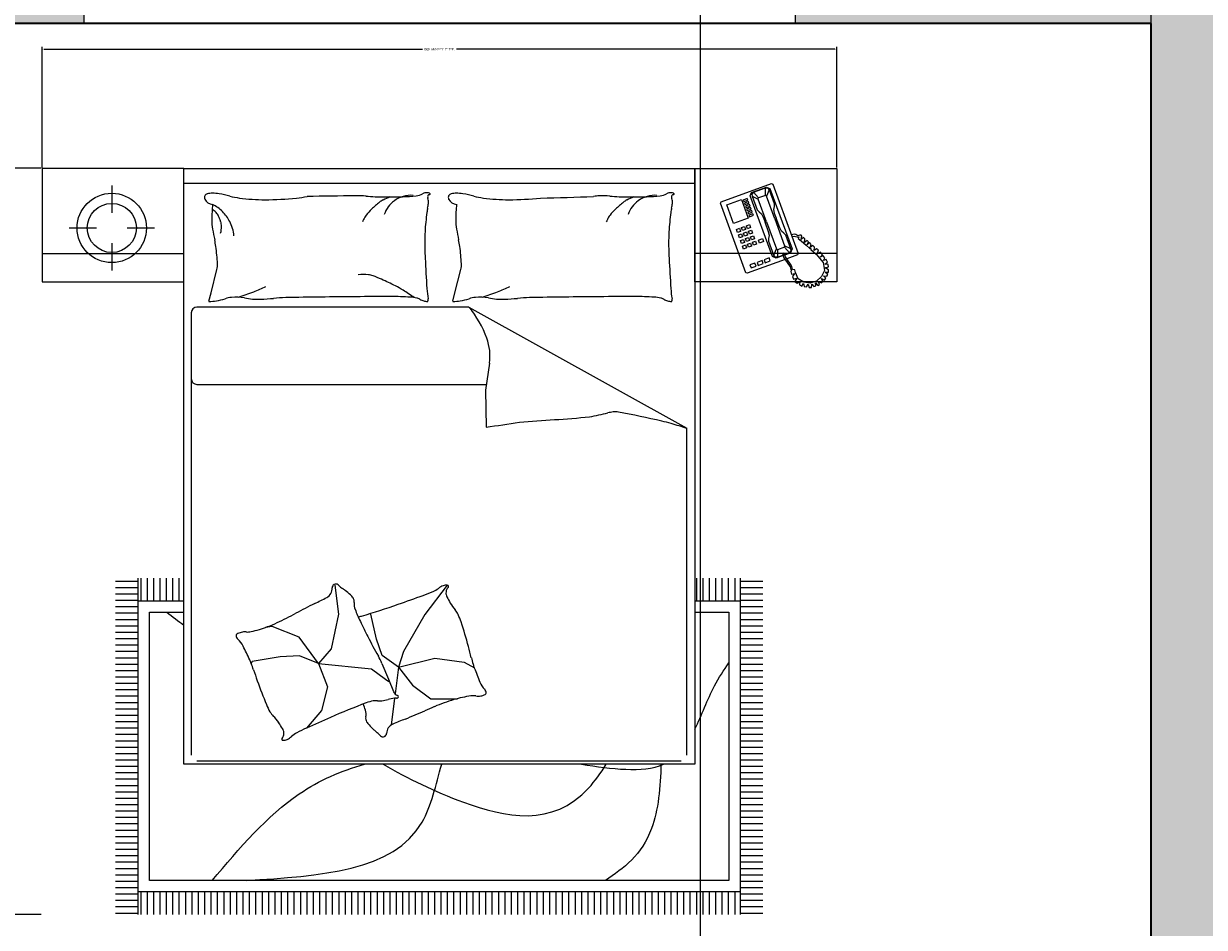
# Model space of a CAD drawing. Units: inches. Extents: x 311 to 815, y -527 to 136.
# Tile 19 of 21: x 444 to 544, y -63 to 13. Entities that reach past the tile are written whole.
import ezdxf

# ---------------------------------------------------------------- set-up
doc = ezdxf.new("R2010")
doc.units = ezdxf.units.IN
doc.header["$MEASUREMENT"] = 0
for name, color, linetype, lineweight in [('A-ANNO-DIMS', 1, 'Continuous', 18), ('A-WALL-PATT', 242, 'Continuous', 13), ('wall', 1, 'Continuous', 35), ('win', 5, 'Continuous', 18)]:
    doc.layers.add(name, color=color, linetype=linetype, lineweight=lineweight)
doc.layers.add('furniture', color=50, linetype='Continuous', lineweight=13, transparency=0.8)
doc.styles.add('DIM_FONT', font='SIMPLEX.shx', dxfattribs={"width": 0.8})
doc.styles.get("Standard").update_dxf_attribs({"font": 'arial.ttf'})
doc.dimstyles.get("Standard").update_dxf_attribs({"dimtxt": 0.18, "dimasz": 0.18, "dimexe": 0.18, "dimexo": 0.0625, "dimgap": 0.09, "dimtad": 0, "dimtih": 1, "dimtoh": 1, "dimdec": 1, "dimzin": 0, "dimdsep": 46, "dimlunit": 4, "dimtxsty": 'Standard', "dimcen": 0.09, "dimadec": 0, "dimazin": 0, "dimtfac": 1, "dimtdec": 1, "dimtofl": 0, "dimtmove": 0, "dimatfit": 3, "dimfxl": 1, "dimtolj": 1, "dimtzin": 0, "dimarcsym": 0})

# ---------------------------------------------------------------- blocks, each defined once
blk = doc.blocks.new('A$C4F634EDD')
for p, q in [((0, 2.6295), (0, 2.2295)), ((0.5, 2.6295), (0, 2.6295)), ((0.5, 2.6295), (2.3, 2.6295)), ((0.5, 0.5295), (0.5, 2.6295)), ((0.5, 2.2295), (0.5, 2.6295)), ((2.3, 2.6295), (2.3, 0.5295)), ((2.3, 2.6295), (2.8, 2.6295)), ((2.3, 2.2295), (2.3, 2.6295)), ((2.8, 2.6295), (2.8, 2.2295)), ((0.2457, 2.5697), (0.2457, 2.4733)), ((0.5, 2.5771), (2.3, 2.5771)), ((2.392, 2.5115), (2.5692, 2.5765)), ((2.4946, 2.5331), (2.4985, 2.5445)), ((2.4985, 2.5445), (2.5516, 2.564)), ((2.5062, 2.5454), (2.5004, 2.5392)), ((2.5004, 2.5392), (2.5013, 2.5315)), ((2.5062, 2.5454), (2.5487, 2.561)), ((2.5235, 2.5256), (2.5062, 2.5454)), ((2.5483, 2.5347), (2.5487, 2.561)), ((2.5487, 2.561), (2.5571, 2.56)), ((2.5615, 2.5536), (2.5514, 2.5318)), ((2.5516, 2.564), (2.5637, 2.5584)), ((2.5571, 2.56), (2.5615, 2.5536)), ((2.5615, 2.5536), (2.5791, 2.5058)), ((2.5637, 2.5584), (2.6418, 2.3458)), ((2.5692, 2.5765), (2.574, 2.5743)), ((2.574, 2.5743), (2.6638, 2.3298)), ((2.3898, 2.5066), (2.392, 2.5115)), ((2.4795, 2.2621), (2.3898, 2.5066)), ((2.412, 2.5007), (2.4634, 2.5196)), ((2.4361, 2.4352), (2.412, 2.5007)), ((2.4634, 2.5196), (2.4875, 2.454)), ((2.4842, 2.5232), (2.47, 2.518)), ((2.47, 2.518), (2.472, 2.5127)), ((2.472, 2.5127), (2.4862, 2.5179)), ((2.4881, 2.5126), (2.4739, 2.5074)), ((2.4739, 2.5074), (2.4759, 2.502)), ((2.4759, 2.502), (2.4901, 2.5073)), ((2.492, 2.5019), (2.4778, 2.4967)), ((2.4778, 2.4967), (2.4798, 2.4914)), ((2.4798, 2.4914), (2.494, 2.4966)), ((2.4862, 2.5179), (2.4842, 2.5232)), ((2.4901, 2.5073), (2.4881, 2.5126)), ((2.494, 2.4966), (2.492, 2.5019)), ((2.5734, 2.3187), (2.4946, 2.5331)), ((2.5013, 2.5315), (2.5188, 2.4836)), ((2.5013, 2.5315), (2.5231, 2.5214)), ((2.5231, 2.5214), (2.5235, 2.5256)), ((2.5523, 2.4417), (2.5231, 2.5214)), ((2.5483, 2.5347), (2.5235, 2.5256)), ((2.5514, 2.5318), (2.5483, 2.5347)), ((2.5807, 2.4521), (2.5514, 2.5318)), ((2.5788, 2.4956), (2.5767, 2.4848)), ((2.5791, 2.5058), (2.5788, 2.4956)), ((2.4875, 2.454), (2.4361, 2.4352)), ((2.4959, 2.4913), (2.4817, 2.4861)), ((2.4817, 2.4861), (2.4837, 2.4808)), ((2.4837, 2.4808), (2.4979, 2.486)), ((2.4998, 2.4807), (2.4856, 2.4755)), ((2.4856, 2.4755), (2.4876, 2.4702)), ((2.4876, 2.4702), (2.5018, 2.4754)), ((2.5037, 2.47), (2.4895, 2.4648)), ((2.4895, 2.4648), (2.4915, 2.4595)), ((2.4915, 2.4595), (2.5057, 2.4647)), ((2.4979, 2.486), (2.4959, 2.4913)), ((2.5018, 2.4754), (2.4998, 2.4807)), ((2.5057, 2.4647), (2.5037, 2.47)), ((2.5188, 2.4836), (2.5256, 2.4761)), ((2.5256, 2.4761), (2.5342, 2.4692)), ((2.5342, 2.4692), (2.5405, 2.4574)), ((2.5405, 2.4574), (2.547, 2.4397)), ((2.5767, 2.4848), (2.5795, 2.4717)), ((2.5795, 2.4717), (2.586, 2.454)), ((2.5984, 2.4204), (2.586, 2.454)), ((0.0957, 2.4197), (0.192, 2.4197)), ((0.2994, 2.4197), (0.3957, 2.4197)), ((2.4457, 2.4146), (2.4563, 2.4185)), ((2.4496, 2.4039), (2.4457, 2.4146)), ((2.4563, 2.4185), (2.4602, 2.4078)), ((2.4634, 2.4211), (2.474, 2.425)), ((2.4673, 2.4104), (2.4634, 2.4211)), ((2.4779, 2.4143), (2.4673, 2.4104)), ((2.474, 2.425), (2.4779, 2.4143)), ((2.4811, 2.4276), (2.4917, 2.4315)), ((2.485, 2.4169), (2.4811, 2.4276)), ((2.4956, 2.4208), (2.485, 2.4169)), ((2.4917, 2.4315), (2.4956, 2.4208)), ((2.5594, 2.4061), (2.547, 2.4397)), ((2.5523, 2.4417), (2.5875, 2.346)), ((2.5807, 2.4521), (2.6158, 2.3564)), ((2.6047, 2.4086), (2.5984, 2.4204)), ((2.4602, 2.4078), (2.4496, 2.4039)), ((2.4528, 2.3951), (2.4635, 2.399)), ((2.4567, 2.3844), (2.4528, 2.3951)), ((2.4674, 2.3883), (2.4567, 2.3844)), ((2.46, 2.3756), (2.4706, 2.3795)), ((2.4639, 2.365), (2.46, 2.3756)), ((2.4635, 2.399), (2.4674, 2.3883)), ((2.4706, 2.4016), (2.4812, 2.4055)), ((2.4745, 2.3909), (2.4706, 2.4016)), ((2.4706, 2.3795), (2.4745, 2.3689)), ((2.4851, 2.3949), (2.4745, 2.3909)), ((2.4777, 2.3821), (2.4883, 2.386)), ((2.4816, 2.3715), (2.4777, 2.3821)), ((2.4812, 2.4055), (2.4851, 2.3949)), ((2.4922, 2.3754), (2.4816, 2.3715)), ((2.4883, 2.4081), (2.4989, 2.412)), ((2.4922, 2.3975), (2.4883, 2.4081)), ((2.4883, 2.386), (2.4922, 2.3754)), ((2.5028, 2.4014), (2.4922, 2.3975)), ((2.4954, 2.3886), (2.5061, 2.3925)), ((2.4993, 2.378), (2.4954, 2.3886)), ((2.4989, 2.412), (2.5028, 2.4014)), ((2.51, 2.3819), (2.4993, 2.378)), ((2.5026, 2.3691), (2.5132, 2.373)), ((2.5061, 2.3925), (2.51, 2.3819)), ((2.5132, 2.373), (2.5171, 2.3624)), ((2.5238, 2.3769), (2.538, 2.3821)), ((2.5277, 2.3663), (2.5238, 2.3769)), ((2.5419, 2.3715), (2.5277, 2.3663)), ((2.538, 2.3821), (2.5419, 2.3715)), ((2.5622, 2.393), (2.5594, 2.4061)), ((2.5598, 2.372), (2.5601, 2.3822)), ((2.5774, 2.3242), (2.5598, 2.372)), ((2.5601, 2.3822), (2.5622, 2.393)), ((2.6133, 2.4017), (2.6047, 2.4086)), ((2.6201, 2.3941), (2.6133, 2.4017)), ((2.6376, 2.3463), (2.6201, 2.3941)), ((2.6499, 2.3979), (2.6397, 2.3953)), ((2.6417, 2.39), (2.6488, 2.391)), ((2.6488, 2.391), (2.6538, 2.3895)), ((2.6551, 2.397), (2.6499, 2.3979)), ((2.6538, 2.3895), (2.6596, 2.388)), ((2.6627, 2.392), (2.6551, 2.397)), ((2.6596, 2.388), (2.6626, 2.3867)), ((2.6626, 2.3867), (2.6662, 2.388)), ((2.6692, 2.394), (2.6627, 2.392)), ((2.6662, 2.388), (2.6632, 2.3828)), ((2.6632, 2.3828), (2.6736, 2.3744)), ((2.6736, 2.3944), (2.6692, 2.394)), ((2.6765, 2.391), (2.6736, 2.3944)), ((2.6736, 2.3744), (2.6922, 2.3593)), ((2.6742, 2.3795), (2.6765, 2.391)), ((2.6824, 2.3858), (2.6742, 2.3795)), ((2.6873, 2.3815), (2.6824, 2.3858)), ((2.6853, 2.369), (2.6873, 2.3815)), ((2.6946, 2.376), (2.6853, 2.369)), ((2.6995, 2.3713), (2.6946, 2.376)), ((2.695, 2.3603), (2.6995, 2.3713)), ((0, 2.3301), (0.5, 2.3301)), ((0.2457, 2.366), (0.2457, 2.2697)), ((2.8, 2.3301), (2.3, 2.3301)), ((2.4745, 2.3689), (2.4639, 2.365)), ((2.4672, 2.3561), (2.4778, 2.36)), ((2.4711, 2.3455), (2.4672, 2.3561)), ((2.4817, 2.3494), (2.4711, 2.3455)), ((2.4778, 2.36), (2.4817, 2.3494)), ((2.4849, 2.3626), (2.4955, 2.3665)), ((2.4888, 2.352), (2.4849, 2.3626)), ((2.4994, 2.3559), (2.4888, 2.352)), ((2.4955, 2.3665), (2.4994, 2.3559)), ((2.5065, 2.3585), (2.5026, 2.3691)), ((2.5171, 2.3624), (2.5065, 2.3585)), ((2.5774, 2.3242), (2.5875, 2.346)), ((2.5875, 2.346), (2.5905, 2.3431)), ((2.5905, 2.3431), (2.5901, 2.3168)), ((2.6154, 2.3522), (2.5905, 2.3431)), ((2.613, 2.3312), (2.6077, 2.3293)), ((2.6077, 2.3293), (2.6135, 2.3141)), ((2.6192, 2.3174), (2.613, 2.3312)), ((2.6153, 2.3261), (2.6327, 2.3324)), ((2.6158, 2.3564), (2.6154, 2.3522)), ((2.6154, 2.3522), (2.6327, 2.3324)), ((2.6376, 2.3463), (2.6158, 2.3564)), ((2.6369, 2.332), (2.6161, 2.3243)), ((2.6327, 2.3324), (2.6385, 2.3386)), ((2.6418, 2.3458), (2.6369, 2.332)), ((2.6385, 2.3386), (2.6376, 2.3463)), ((2.6638, 2.3298), (2.6616, 2.3249)), ((2.6922, 2.3593), (2.7051, 2.3473)), ((2.7031, 2.3682), (2.695, 2.3603)), ((2.7096, 2.3616), (2.7031, 2.3682)), ((2.7051, 2.3473), (2.7079, 2.3475)), ((2.7062, 2.351), (2.7096, 2.3616)), ((2.7147, 2.3578), (2.7062, 2.351)), ((2.7079, 2.3475), (2.7079, 2.3443)), ((2.7079, 2.3443), (2.727, 2.3277)), ((2.7214, 2.3517), (2.7147, 2.3578)), ((2.7196, 2.34), (2.7214, 2.3517)), ((2.7286, 2.3466), (2.7196, 2.34)), ((2.7346, 2.3423), (2.7286, 2.3466)), ((2.732, 2.3295), (2.7346, 2.3423)), ((2.7423, 2.3345), (2.732, 2.3295)), ((2.7495, 2.325), (2.7423, 2.3345)), ((2.6172, 2.3086), (2.4844, 2.2599)), ((2.5114, 2.2959), (2.4936, 2.2894)), ((2.4936, 2.2894), (2.4976, 2.2788)), ((2.5153, 2.2853), (2.5114, 2.2959)), ((2.5362, 2.305), (2.5185, 2.2985)), ((2.5185, 2.2985), (2.5224, 2.2879)), ((2.5224, 2.2879), (2.5401, 2.2944)), ((2.5401, 2.2944), (2.5362, 2.305)), ((2.561, 2.3141), (2.5433, 2.3076)), ((2.5433, 2.3076), (2.5472, 2.297)), ((2.5472, 2.297), (2.5649, 2.3035)), ((2.5649, 2.3035), (2.561, 2.3141)), ((2.5855, 2.3131), (2.5734, 2.3187)), ((2.5818, 2.3178), (2.5774, 2.3242)), ((2.5901, 2.3168), (2.5818, 2.3178)), ((2.6104, 2.3222), (2.5855, 2.3131)), ((2.5901, 2.3168), (2.6097, 2.324)), ((2.6135, 2.3141), (2.6244, 2.2977)), ((2.626, 2.3069), (2.6192, 2.3174)), ((2.6616, 2.3249), (2.6234, 2.3109)), ((2.6244, 2.2977), (2.6349, 2.2825)), ((2.6365, 2.2916), (2.626, 2.3069)), ((2.6407, 2.2834), (2.6365, 2.2916)), ((2.727, 2.3277), (2.7512, 2.2983)), ((2.7406, 2.3172), (2.7495, 2.325)), ((2.7519, 2.3218), (2.7406, 2.3172)), ((2.7512, 2.2983), (2.756, 2.2695)), ((2.7575, 2.3144), (2.7519, 2.3218)), ((2.7526, 2.3045), (2.7575, 2.3144)), ((2.7622, 2.308), (2.7526, 2.3045)), ((2.7574, 2.2924), (2.7673, 2.2997)), ((2.7687, 2.2905), (2.7574, 2.2924)), ((2.7673, 2.2997), (2.7622, 2.308)), ((2.7699, 2.2828), (2.7687, 2.2905)), ((0.5953, 2.1912), (0.616, 2.2738)), ((1.4546, 2.1912), (1.4752, 2.2738)), ((2.4844, 2.2599), (2.4795, 2.2621)), ((2.4976, 2.2788), (2.5153, 2.2853)), ((2.6349, 2.2825), (2.638, 2.273)), ((2.6399, 2.2712), (2.6374, 2.2659)), ((2.6374, 2.2659), (2.6398, 2.257)), ((2.638, 2.273), (2.6399, 2.2712)), ((2.6398, 2.257), (2.6509, 2.259)), ((2.6438, 2.2739), (2.6407, 2.2834)), ((2.6509, 2.259), (2.6431, 2.2492)), ((2.6431, 2.2492), (2.6473, 2.2398)), ((2.6519, 2.2716), (2.6438, 2.2739)), ((2.6535, 2.2628), (2.6519, 2.2716)), ((2.6636, 2.2409), (2.6535, 2.2628)), ((2.7459, 2.2483), (2.7284, 2.2317)), ((2.756, 2.2695), (2.7459, 2.2483)), ((2.7529, 2.2505), (2.7645, 2.2498)), ((2.7607, 2.2424), (2.7529, 2.2505)), ((2.7587, 2.279), (2.7699, 2.2828)), ((2.7708, 2.2725), (2.7587, 2.279)), ((2.759, 2.2637), (2.7706, 2.2643)), ((2.7676, 2.2559), (2.759, 2.2637)), ((2.7645, 2.2498), (2.7676, 2.2559)), ((2.7706, 2.2643), (2.7708, 2.2725)), ((0, 2.2295), (0.5, 2.2295)), ((2.8, 2.2295), (2.3, 2.2295)), ((2.6473, 2.2398), (2.6592, 2.2429)), ((2.6592, 2.2429), (2.6521, 2.2314)), ((2.6521, 2.2314), (2.6598, 2.2248)), ((2.6598, 2.2248), (2.6697, 2.2309)), ((2.6836, 2.2287), (2.6636, 2.2409)), ((2.6697, 2.2309), (2.6684, 2.219)), ((2.6684, 2.219), (2.6761, 2.2145)), ((2.6761, 2.2145), (2.6821, 2.2237)), ((2.6821, 2.2237), (2.6843, 2.2135)), ((2.7063, 2.2256), (2.6836, 2.2287)), ((2.6843, 2.2135), (2.6927, 2.2117)), ((2.6927, 2.2117), (2.6986, 2.222)), ((2.6986, 2.222), (2.7019, 2.2098)), ((2.7019, 2.2098), (2.7102, 2.2104)), ((2.7284, 2.2317), (2.7063, 2.2256)), ((2.7102, 2.2104), (2.7113, 2.2218)), ((2.7113, 2.2218), (2.7192, 2.2137)), ((2.7192, 2.2137), (2.7255, 2.2152)), ((2.7255, 2.2152), (2.7242, 2.2265)), ((2.7242, 2.2265), (2.7324, 2.2165)), ((2.7324, 2.2165), (2.7386, 2.2208)), ((2.7386, 2.2208), (2.7354, 2.2306)), ((2.7354, 2.2306), (2.7462, 2.2264)), ((2.7509, 2.2314), (2.7459, 2.2418)), ((2.7459, 2.2418), (2.7568, 2.2352)), ((2.7462, 2.2264), (2.7509, 2.2314)), ((2.7568, 2.2352), (2.7607, 2.2424)), ((0.5878, 2.1612), (0.5953, 2.1912)), ((1.4471, 2.1612), (1.4546, 2.1912)), ((1.5035, 2.141), (0.5458, 2.141)), ((1.5035, 2.141), (2.2716, 1.7136)), ((0.5258, 2.121), (0.5258, 0.5617)), ((1.576, 1.9433), (1.5624, 1.8479)), ((0.5458, 1.8684), (1.5653, 1.8684)), ((1.5624, 1.8479), (1.5641, 1.7178)), ((2.2716, 0.5617), (2.2716, 1.7136)), ((0.2586, 1.1753), (0.3386, 1.1753)), ((0.3386, 0), (0.3386, 1.1852)), ((0.3486, 1.1052), (0.3486, 1.1852)), ((0.3711, 1.1052), (0.3711, 1.1852)), ((0.3936, 1.1052), (0.3936, 1.1852)), ((0.4161, 1.1052), (0.4161, 1.1852)), ((0.4386, 1.1052), (0.4386, 1.1852)), ((0.4611, 1.1052), (0.4611, 1.1852)), ((0.4836, 1.1052), (0.4836, 1.1852)), ((2.3061, 1.1052), (2.3061, 1.1852)), ((2.3286, 1.1052), (2.3286, 1.1852)), ((2.3511, 1.1052), (2.3511, 1.1852)), ((2.3736, 1.1052), (2.3736, 1.1852)), ((2.3961, 1.1052), (2.3961, 1.1852)), ((2.4186, 1.1052), (2.4186, 1.1852)), ((2.4411, 1.1052), (2.4411, 1.1852)), ((2.4588, 1.1852), (2.4588, 0)), ((2.4588, 1.1753), (2.5388, 1.1753)), ((0.2586, 1.1528), (0.3386, 1.1528)), ((0.2586, 1.1303), (0.3386, 1.1303)), ((1.031, 1.1612), (1.0448, 1.0581)), ((1.4276, 1.1611), (1.3484, 1.0571)), ((2.4588, 1.1528), (2.5388, 1.1528)), ((2.4588, 1.1303), (2.5388, 1.1303)), ((0.2586, 1.1078), (0.3386, 1.1078)), ((0.2586, 1.0853), (0.3386, 1.0853)), ((0.3386, 1.1052), (0.5, 1.1052)), ((2.3, 1.1052), (2.4588, 1.1052)), ((2.4588, 1.1078), (2.5388, 1.1078)), ((2.4588, 1.0853), (2.5388, 1.0853)), ((0.2586, 1.0628), (0.3386, 1.0628)), ((0.2586, 1.0403), (0.3386, 1.0403)), ((0.3786, 1.0652), (0.5, 1.0652)), ((0.3786, 0.12), (0.3786, 1.0652)), ((1.0448, 1.0581), (1.019, 0.936)), ((1.1784, 0.9702), (1.1586, 1.0591)), ((1.3484, 1.0571), (1.2733, 0.9268)), ((2.3, 1.0652), (2.4188, 1.0652)), ((2.4188, 1.0652), (2.4188, 0.12)), ((2.4588, 1.0628), (2.5388, 1.0628)), ((2.4588, 1.0403), (2.5388, 1.0403)), ((0.2586, 1.0178), (0.3386, 1.0178)), ((0.8108, 1.0151), (0.7868, 1.0117)), ((0.9054, 0.9773), (0.8108, 1.0151)), ((2.4588, 1.0178), (2.5388, 1.0178)), ((0.2586, 0.9953), (0.3386, 0.9953)), ((0.2586, 0.9728), (0.3386, 0.9728)), ((0.9743, 0.8845), (0.9054, 0.9773)), ((1.1982, 0.9129), (1.1784, 0.9702)), ((2.4588, 0.9953), (2.5388, 0.9953)), ((2.4588, 0.9728), (2.5388, 0.9728)), ((0.2586, 0.9503), (0.3386, 0.9503)), ((0.2586, 0.9278), (0.3386, 0.9278)), ((1.019, 0.936), (0.9743, 0.8845)), ((1.2733, 0.9268), (1.2555, 0.8715)), ((2.4588, 0.9503), (2.5388, 0.9503)), ((2.4588, 0.9278), (2.5388, 0.9278)), ((0.2586, 0.9053), (0.3386, 0.9053)), ((0.2586, 0.8828), (0.3386, 0.8828)), ((0.7403, 0.8913), (0.737, 0.8849)), ((0.8384, 0.9085), (0.7403, 0.8913)), ((0.9072, 0.912), (0.8384, 0.9085)), ((0.9743, 0.8845), (0.9072, 0.912)), ((0.9743, 0.8845), (1.0052, 0.802)), ((0.9743, 0.8845), (1.16, 0.8656)), ((1.1973, 0.8853), (1.2203, 0.829)), ((1.2555, 0.8715), (1.1982, 0.9129)), ((1.2555, 0.8715), (1.384, 0.9031)), ((1.384, 0.9031), (1.4868, 0.8892)), ((1.4868, 0.8892), (1.5228, 0.8692)), ((2.4588, 0.9053), (2.5388, 0.9053)), ((2.4588, 0.8828), (2.5388, 0.8828)), ((0.2586, 0.8603), (0.3386, 0.8603)), ((0.2586, 0.8378), (0.3386, 0.8378)), ((1.16, 0.8656), (1.2099, 0.8295)), ((1.2555, 0.8715), (1.2437, 0.7773)), ((1.2555, 0.8715), (1.3049, 0.8082)), ((2.4588, 0.8603), (2.5388, 0.8603)), ((2.4588, 0.8378), (2.5388, 0.8378)), ((0.2586, 0.8153), (0.3386, 0.8153)), ((0.2586, 0.7928), (0.3386, 0.7928)), ((1.0052, 0.802), (0.9846, 0.7194)), ((1.2099, 0.8295), (1.222, 0.8209)), ((1.2203, 0.829), (1.2381, 0.7855)), ((1.3049, 0.8082), (1.3701, 0.7608)), ((2.4588, 0.8153), (2.5388, 0.8153)), ((2.4588, 0.7928), (2.5388, 0.7928)), ((0.2586, 0.7703), (0.3386, 0.7703)), ((1.2419, 0.7626), (1.23, 0.668)), ((1.3701, 0.7608), (1.463, 0.7608)), ((2.4588, 0.7703), (2.5388, 0.7703)), ((0.2586, 0.7478), (0.3386, 0.7478)), ((0.2586, 0.7253), (0.3386, 0.7253)), ((0.9846, 0.7194), (0.931, 0.6569)), ((2.4588, 0.7478), (2.5388, 0.7478)), ((2.4588, 0.7253), (2.5388, 0.7253)), ((0.2586, 0.7028), (0.3386, 0.7028)), ((0.2586, 0.6803), (0.3386, 0.6803)), ((2.4588, 0.7028), (2.5388, 0.7028)), ((2.4588, 0.6803), (2.5388, 0.6803)), ((0.2586, 0.6578), (0.3386, 0.6578)), ((0.2586, 0.6353), (0.3386, 0.6353)), ((2.4588, 0.6578), (2.5388, 0.6578)), ((2.4588, 0.6353), (2.5388, 0.6353)), ((0.2586, 0.6128), (0.3386, 0.6128)), ((0.2586, 0.5903), (0.3386, 0.5903)), ((2.4588, 0.6128), (2.5388, 0.6128)), ((2.4588, 0.5903), (2.5388, 0.5903)), ((0.2586, 0.5678), (0.3386, 0.5678)), ((0.2586, 0.5453), (0.3386, 0.5453)), ((0.5458, 0.5417), (2.2516, 0.5417)), ((2.4588, 0.5678), (2.5388, 0.5678)), ((2.4588, 0.5453), (2.5388, 0.5453)), ((0.2586, 0.5228), (0.3386, 0.5228)), ((0.2586, 0.5003), (0.3386, 0.5003)), ((2.3, 0.5295), (0.5, 0.5295)), ((2.4588, 0.5228), (2.5388, 0.5228)), ((2.4588, 0.5003), (2.5388, 0.5003)), ((0.2586, 0.4778), (0.3386, 0.4778)), ((2.4588, 0.4778), (2.5388, 0.4778)), ((0.2586, 0.4553), (0.3386, 0.4553)), ((0.2586, 0.4328), (0.3386, 0.4328)), ((2.4588, 0.4553), (2.5388, 0.4553)), ((2.4588, 0.4328), (2.5388, 0.4328)), ((0.2586, 0.4103), (0.3386, 0.4103)), ((0.2586, 0.3878), (0.3386, 0.3878)), ((2.4588, 0.4103), (2.5388, 0.4103)), ((2.4588, 0.3878), (2.5388, 0.3878)), ((0.2586, 0.3653), (0.3386, 0.3653)), ((0.2586, 0.3428), (0.3386, 0.3428)), ((2.4588, 0.3653), (2.5388, 0.3653)), ((2.4588, 0.3428), (2.5388, 0.3428)), ((0.2586, 0.3203), (0.3386, 0.3203)), ((0.2586, 0.2978), (0.3386, 0.2978)), ((2.4588, 0.3203), (2.5388, 0.3203)), ((2.4588, 0.2978), (2.5388, 0.2978)), ((0.2586, 0.2753), (0.3386, 0.2753)), ((0.2586, 0.2528), (0.3386, 0.2528)), ((2.4588, 0.2753), (2.5388, 0.2753)), ((2.4588, 0.2528), (2.5388, 0.2528)), ((0.2586, 0.2303), (0.3386, 0.2303)), ((2.4588, 0.2303), (2.5388, 0.2303)), ((0.2586, 0.2078), (0.3386, 0.2078)), ((0.2586, 0.1853), (0.3386, 0.1853)), ((2.4588, 0.2078), (2.5388, 0.2078)), ((2.4588, 0.1853), (2.5388, 0.1853)), ((0.2586, 0.1628), (0.3386, 0.1628)), ((0.2586, 0.1403), (0.3386, 0.1403)), ((2.4588, 0.1628), (2.5388, 0.1628)), ((2.4588, 0.1403), (2.5388, 0.1403)), ((0.2586, 0.1178), (0.3386, 0.1178)), ((0.2586, 0.0953), (0.3386, 0.0953)), ((2.4188, 0.12), (0.3786, 0.12)), ((2.4588, 0.1178), (2.5388, 0.1178)), ((2.4588, 0.0953), (2.5388, 0.0953)), ((0.2586, 0.0728), (0.3386, 0.0728)), ((0.2586, 0.0503), (0.3386, 0.0503)), ((2.4588, 0.08), (0.3386, 0.08)), ((0.3486, 0), (0.3486, 0.08)), ((0.3711, 0), (0.3711, 0.08)), ((0.3936, 0), (0.3936, 0.08)), ((0.4161, 0), (0.4161, 0.08)), ((0.4386, 0), (0.4386, 0.08)), ((0.4611, 0), (0.4611, 0.08)), ((0.4836, 0), (0.4836, 0.08)), ((0.5061, 0), (0.5061, 0.08)), ((0.5286, 0), (0.5286, 0.08)), ((0.5511, 0), (0.5511, 0.08)), ((0.5736, 0), (0.5736, 0.08)), ((0.5961, 0), (0.5961, 0.08)), ((0.6186, 0), (0.6186, 0.08)), ((0.6411, 0), (0.6411, 0.08)), ((0.6636, 0), (0.6636, 0.08)), ((0.6861, 0), (0.6861, 0.08)), ((0.7086, 0), (0.7086, 0.08)), ((0.7311, 0), (0.7311, 0.08)), ((0.7536, 0), (0.7536, 0.08)), ((0.7761, 0), (0.7761, 0.08)), ((0.7986, 0), (0.7986, 0.08)), ((0.8211, 0), (0.8211, 0.08)), ((0.8436, 0), (0.8436, 0.08)), ((0.8661, 0), (0.8661, 0.08)), ((0.8886, 0), (0.8886, 0.08)), ((0.9111, 0), (0.9111, 0.08)), ((0.9336, 0), (0.9336, 0.08)), ((0.9561, 0), (0.9561, 0.08)), ((0.9786, 0), (0.9786, 0.08)), ((1.0011, 0), (1.0011, 0.08)), ((1.0236, 0), (1.0236, 0.08)), ((1.0461, 0), (1.0461, 0.08)), ((1.0686, 0), (1.0686, 0.08)), ((1.0911, 0), (1.0911, 0.08)), ((1.1136, 0), (1.1136, 0.08)), ((1.1361, 0), (1.1361, 0.08)), ((1.1586, 0), (1.1586, 0.08)), ((1.1811, 0), (1.1811, 0.08)), ((1.2036, 0), (1.2036, 0.08)), ((1.2261, 0), (1.2261, 0.08)), ((1.2486, 0), (1.2486, 0.08)), ((1.2711, 0), (1.2711, 0.08)), ((1.2936, 0), (1.2936, 0.08)), ((1.3161, 0), (1.3161, 0.08)), ((1.3386, 0), (1.3386, 0.08)), ((1.3611, 0), (1.3611, 0.08)), ((1.3836, 0), (1.3836, 0.08)), ((1.4061, 0), (1.4061, 0.08)), ((1.4286, 0), (1.4286, 0.08)), ((1.4511, 0), (1.4511, 0.08)), ((1.4736, 0), (1.4736, 0.08)), ((1.4961, 0), (1.4961, 0.08)), ((1.5186, 0), (1.5186, 0.08)), ((1.5411, 0), (1.5411, 0.08)), ((1.5636, 0), (1.5636, 0.08)), ((1.5861, 0), (1.5861, 0.08)), ((1.6086, 0), (1.6086, 0.08)), ((1.6311, 0), (1.6311, 0.08)), ((1.6536, 0), (1.6536, 0.08)), ((1.6761, 0), (1.6761, 0.08)), ((1.6986, 0), (1.6986, 0.08)), ((1.7211, 0), (1.7211, 0.08)), ((1.7436, 0), (1.7436, 0.08)), ((1.7661, 0), (1.7661, 0.08)), ((1.7886, 0), (1.7886, 0.08)), ((1.8111, 0), (1.8111, 0.08)), ((1.8336, 0), (1.8336, 0.08)), ((1.8561, 0), (1.8561, 0.08)), ((1.8786, 0), (1.8786, 0.08)), ((1.9011, 0), (1.9011, 0.08)), ((1.9236, 0), (1.9236, 0.08)), ((1.9461, 0), (1.9461, 0.08)), ((1.9686, 0), (1.9686, 0.08)), ((1.9911, 0), (1.9911, 0.08)), ((2.0136, 0), (2.0136, 0.08)), ((2.0361, 0), (2.0361, 0.08)), ((2.0586, 0), (2.0586, 0.08)), ((2.0811, 0), (2.0811, 0.08)), ((2.1036, 0), (2.1036, 0.08)), ((2.1261, 0), (2.1261, 0.08)), ((2.1486, 0), (2.1486, 0.08)), ((2.1711, 0), (2.1711, 0.08)), ((2.1936, 0), (2.1936, 0.08)), ((2.2161, 0), (2.2161, 0.08)), ((2.2386, 0), (2.2386, 0.08)), ((2.2611, 0), (2.2611, 0.08)), ((2.2836, 0), (2.2836, 0.08)), ((2.3061, 0), (2.3061, 0.08)), ((2.3286, 0), (2.3286, 0.08)), ((2.3511, 0), (2.3511, 0.08)), ((2.3736, 0), (2.3736, 0.08)), ((2.3961, 0), (2.3961, 0.08)), ((2.4186, 0), (2.4186, 0.08)), ((2.4411, 0), (2.4411, 0.08)), ((2.4588, 0.0728), (2.5388, 0.0728)), ((2.4588, 0.0503), (2.5388, 0.0503)), ((0.2586, 0.0278), (0.3386, 0.0278)), ((0.2586, 0.0053), (0.3386, 0.0053)), ((2.4588, 0.0278), (2.5388, 0.0278)), ((2.4588, 0.0053), (2.5388, 0.0053))]:
    blk.add_line(p, q)
for radius in [0.1222, 0.0865]:
    blk.add_circle((0.2457, 2.4197), radius)
for centre, radius, start, end in [((0.5848, 2.5274), 0.0131, 101.2724, 206.5805), ((0.5999, 2.4516), 0.0904, 90, 101.2724), ((0.5999, 2.3808), 0.1611, 81.5628, 90), ((0.5788, 2.2388), 0.3048, 74.256, 81.5628), ((1.3132, 2.5864), 0.0539, 275.2592, 300.6513), ((1.3554, 2.5152), 0.0289, 85.6975, 120.6513), ((1.3556, 2.519), 0.0251, 68.2117, 85.6975), ((1.3634, 2.533), 0.00428, 78.1069, 158.0096), ((1.3647, 2.5395), 0.00232, 258.1069, 19.564), ((1.3637, 2.5391), 0.00342, 19.564, 68.2117), ((1.444, 2.5274), 0.0131, 101.2724, 206.5805), ((1.4591, 2.4516), 0.0904, 90, 101.2724), ((1.4591, 2.3808), 0.1611, 81.5628, 90), ((1.438, 2.2388), 0.3048, 74.256, 81.5628), ((2.1724, 2.5864), 0.0539, 275.2592, 300.6513), ((2.2146, 2.5152), 0.0289, 85.6975, 120.6513), ((2.2149, 2.519), 0.0251, 68.2117, 85.6975), ((2.2226, 2.533), 0.00428, 78.1069, 158.0096), ((2.224, 2.5395), 0.00232, 258.1069, 19.564), ((2.2229, 2.5391), 0.00342, 19.564, 68.2117), ((0.6036, 2.5368), 0.0342, 206.5805, 265.5998), ((1.0898, 2.4496), 0.4918, 173.7676, 180), ((0.5368, 2.3783), 0.1399, 45.0976, 62.7964), ((0.7272, 2.7653), 0.2422, 254.256, 262.4531), ((0.7851, 3.2019), 0.6827, 262.4531, 270), ((0.7851, 3.5682), 1.049, 270, 276.0867), ((0.8402, 3.0514), 0.5293, 276.0867, 280.1899), ((1.1602, -8.1346), 10.6675, 90.30153, 91.21582), ((1.1169, 2.2433), 0.2897, 85.1982, 92.5386), ((1.2142, 3.4021), 0.8732, 265.1982, 269.4243), ((1.4317, 2.2032), 0.3916, 128.3886, 133.8115), ((1.2362, 2.45), 0.0768, 117.2396, 128.3886), ((1.3082, 2.3102), 0.234, 110.8603, 117.2396), ((1.2204, 4.0232), 1.4943, 269.4243, 271.9079), ((1.2995, 2.4357), 0.0992, 126.0864, 143.8234), ((1.2995, 2.4357), 0.0992, 105.9352, 126.0864), ((1.2429, 3.3501), 0.8208, 271.9079, 275.2592), ((1.2995, 2.4357), 0.0992, 85.7841, 105.9352), ((1.3739, 2.5288), 0.0156, 158.0096, 201.421), ((1.1177, 2.5413), 0.246, 347.8905, 351.8665), ((1.3288, 2.5111), 0.0328, 351.8665, 21.421), ((1.4628, 2.5368), 0.0342, 206.5805, 265.5998), ((1.949, 2.4496), 0.4918, 173.7676, 180), ((1.5865, 2.7653), 0.2422, 254.256, 262.4531), ((1.6443, 3.2019), 0.6827, 262.4531, 270), ((1.6443, 3.5682), 1.049, 270, 276.0867), ((1.4785, 15.4878), 12.9656, 271.22425, 272.05324), ((1.97, 2.3805), 0.1524, 92.5386, 100.1899), ((1.9761, 2.2433), 0.2897, 85.1982, 92.5386), ((2.0734, 3.4021), 0.8732, 265.1982, 269.4243), ((2.291, 2.2032), 0.3916, 128.3886, 133.8115), ((2.0954, 2.45), 0.0768, 117.2396, 128.3886), ((2.1674, 2.3102), 0.234, 110.8603, 117.2396), ((2.0797, 4.0232), 1.4943, 269.4243, 271.9079), ((2.1588, 2.4357), 0.0992, 126.0864, 143.8234), ((2.1588, 2.4357), 0.0992, 105.9352, 126.0864), ((2.1021, 3.3501), 0.8208, 271.9079, 275.2592), ((2.1588, 2.4357), 0.0992, 85.7841, 105.9352), ((2.2331, 2.5288), 0.0156, 158.0096, 201.421), ((1.977, 2.5413), 0.246, 347.8905, 351.8665), ((2.1881, 2.5111), 0.0328, 351.8665, 21.421), ((0.5462, 2.4142), 0.0899, 41.4429, 53.7359), ((0.5741, 2.4389), 0.0526, 25.3551, 41.4429), ((0.4851, 2.3967), 0.1511, 21.8149, 25.3551), ((0.5368, 2.3783), 0.1399, 27.3988, 45.0976), ((1.3127, 2.3625), 0.2002, 151.6832, 156.9972), ((1.1799, 2.4341), 0.0493, 140.9651, 151.6832), ((1.3165, 2.3233), 0.2252, 133.8115, 140.9651), ((1.2995, 2.4357), 0.0992, 143.8234, 161.5603), ((2.2605, 2.3525), 0.9131, 172.3191, 176.6313), ((1.5522, 2.448), 0.1983, 167.8905, 172.3191), ((2.1719, 2.3625), 0.2002, 151.6832, 156.9972), ((2.0391, 2.4341), 0.0493, 140.9651, 151.6832), ((2.1757, 2.3233), 0.2252, 133.8115, 140.9651), ((2.1588, 2.4357), 0.0992, 143.8234, 161.5603), ((3.1198, 2.3525), 0.9131, 172.3191, 176.6313), ((2.4114, 2.448), 0.1983, 167.8905, 172.3191), ((0.8019, 2.4496), 0.204, 180, 189.6844), ((1.4703, 2.5637), 0.882, 189.6844, 192.1984), ((0.4345, 2.3765), 0.2056, 18.7799, 21.8149), ((0.576, 2.4246), 0.0562, 0, 18.7799), ((0.5406, 2.4246), 0.0915, 345.3149, 0), ((0.5368, 2.3783), 0.1399, 16.515, 27.3988), ((0.5368, 2.3783), 0.1399, 5.6311, 16.515), ((1.6611, 2.4496), 0.204, 180, 189.6844), ((2.3295, 2.5637), 0.882, 189.6844, 192.1984), ((0.2982, 2.3103), 0.3171, 8.0051, 12.1984), ((2.0266, 2.3663), 0.6787, 176.6313, 181.6331), ((1.1575, 2.3103), 0.3171, 8.0051, 12.1984), ((2.8858, 2.3663), 0.6787, 176.6313, 181.6331), ((-0.0401, 2.2627), 0.6588, 2.6649, 8.0051), ((2.7128, 2.3859), 1.3652, 181.6331, 183.055), ((0.8191, 2.2627), 0.6588, 2.6649, 8.0051), ((3.5721, 2.3859), 1.3652, 181.6331, 183.055), ((0.5503, 2.2902), 0.0677, 345.9548, 2.6649), ((14.9657, 3.0398), 13.6356, 183.05496, 183.50486), ((1.4096, 2.2902), 0.0677, 345.9548, 2.6649), ((15.8249, 3.0398), 13.6356, 183.05496, 183.50486), ((1.1303, 1.9835), 0.2721, 85.9172, 93.5552), ((1.1455, 2.197), 0.058, 69.3257, 85.9172), ((0.9871, 1.7772), 0.5066, 65.6735, 69.3257), ((0.473, 2.8815), 0.7387, 293.4844, 295.3111), ((0.6058, 0.9338), 1.4323, 63.5015, 65.6735), ((1.1054, 1.9358), 0.3126, 57.865, 63.5015), ((1.6762, 2.2258), 0.3212, 183.5049, 189.9984), ((1.3322, 2.8815), 0.7387, 293.4844, 295.3111), ((2.5355, 2.2258), 0.3212, 183.5049, 189.9984), ((0.5695, 2.4301), 0.2708, 274.0829, 279.4841), ((0.5763, 2.3896), 0.2297, 279.4841, 287.3864), ((0.6807, 2.0561), 0.1197, 96.4341, 107.3864), ((0.6836, 2.0301), 0.1459, 78.4414, 96.4341), ((0.473, 2.8815), 0.7387, 287.1982, 289.428), ((0.759, 2.3985), 0.2301, 258.4414, 272.7491), ((0.473, 2.8815), 0.7387, 289.428, 291.6577), ((0.473, 2.8815), 0.7387, 291.6577, 293.4844), ((0.7026, 3.5718), 1.4048, 272.7491, 274.6176), ((0.9136, 0.9591), 1.2165, 92.6096, 94.6176), ((1.2501, -19.8405), 22.0183, 90.37908, 91.01965), ((1.2012, -3.5404), 5.7185, 89.7135, 90.9704), ((1.224, 1.0141), 1.164, 86.426, 89.7135), ((0.8841, 1.5835), 0.7286, 54.1737, 57.865), ((1.2875, 2.0302), 0.1459, 77.131, 86.426), ((1.3099, 2.1283), 0.0453, 62.7159, 77.131), ((1.3658, 2.2367), 0.0767, 242.7159, 253.7788), ((1.3688, 2.247), 0.0875, 253.7788, 262.8796), ((1.3409, 2.1667), 0.0193, 343.3022, 9.9984), ((1.4288, 2.4301), 0.2708, 274.0829, 279.4841), ((1.4355, 2.3896), 0.2297, 279.4841, 287.3864), ((1.5399, 2.0561), 0.1197, 96.4341, 107.3864), ((1.5429, 2.0301), 0.1459, 78.4414, 96.4341), ((1.3322, 2.8815), 0.7387, 287.1982, 289.428), ((1.6182, 2.3985), 0.2301, 258.4414, 272.7491), ((1.3322, 2.8815), 0.7387, 289.428, 291.6577), ((1.3322, 2.8815), 0.7387, 291.6577, 293.4844), ((1.5619, 3.5718), 1.4048, 272.7491, 274.6176), ((1.7729, 0.9591), 1.2165, 92.6096, 94.6176), ((2.1093, -19.8405), 22.0183, 90.37908, 91.01965), ((2.0605, -3.5404), 5.7185, 89.7135, 90.9704), ((2.0833, 1.0141), 1.164, 86.426, 89.7135), ((2.1467, 2.0302), 0.1459, 77.131, 86.426), ((2.1691, 2.1283), 0.0453, 62.7159, 77.131), ((2.2251, 2.2367), 0.0767, 242.7159, 253.7788), ((2.2281, 2.247), 0.0875, 253.7788, 262.8796), ((2.2001, 2.1667), 0.0193, 343.3022, 9.9984), ((0.5458, 2.121), 0.02, 90, 180), ((0.5887, 2.1609), 0.000917, 165.9551, 274.0829), ((1.3581, 2.1615), 0.00132, 262.8796, 343.3022), ((1.448, 2.1609), 0.000917, 165.9551, 274.0829), ((1.2147, 1.9017), 0.3751, 20.1488, 39.6445), ((2.2174, 2.1615), 0.00132, 262.8796, 343.3022), ((1.3977, 1.9688), 0.1801, 351.8644, 20.1488), ((0.5458, 1.8884), 0.02, 180, 270), ((0.6102, 18.0525), 16.3521, 273.75703, 274.62393), ((1.4194, 4.2174), 2.5158, 281.6741, 283.1904), ((2.0378, 1.5789), 0.1942, 97.7304, 103.1904), ((2.0195, 1.7137), 0.0581, 79.2724, 97.7304), ((1.2737, -2.2227), 4.0646, 77.0745, 79.2724), ((1.0582, 5.4638), 3.7801, 277.692, 279.495), ((2.0359, 1.0981), 0.6574, 74.0648, 77.0745), ((1.7125, -0.0344), 1.8351, 72.2636, 74.0648), ((1.0348, 1.1521), 0.0127, 51.1864, 183.2455), ((0.9863, 1.1494), 0.0359, 297.2902, 3.2455), ((0.9991, 1.1077), 0.0697, 45.8726, 51.1864), ((1.0791, 1.1902), 0.0452, 225.8726, 232.4713), ((1.2846, 1.4577), 0.3825, 232.4713, 233.7837), ((0.6683, 0.6162), 0.6605, 52.7849, 53.7837), ((0.9362, 0.9689), 0.2176, 46.4776, 52.7849), ((1.0327, 1.0706), 0.0774, 35.8936, 46.4776), ((-0.4107, 5.9078), 5.0942, 289.0836, 290.1287), ((1.0543, 1.9106), 0.8371, 290.1287, 292.7069), ((1.3469, 1.2115), 0.0792, 292.7069, 308.5854), ((1.4338, 1.1026), 0.0601, 110.3452, 128.5854), ((1.4251, 1.1259), 0.0352, 86.0516, 110.3452), ((1.4996, 1.1284), 0.0771, 169.5926, 177.2714), ((1.4378, 1.1314), 0.0153, 177.2714, 194.5709), ((1.4611, 1.1374), 0.0393, 194.5709, 206.8179), ((1.4376, 1.1398), 0.0142, 126.5792, 169.5926), ((1.4273, 1.1567), 0.00443, 13.2808, 86.0516), ((1.4254, 1.1562), 0.0063, 306.5792, 13.2808), ((1.8575, -0.7096), 2.0162, 116.4147, 117.4999), ((-0.4173, 3.8699), 3.0972, 296.4147, 297.2902), ((1.0771, 1.1027), 0.0226, 351.9508, 35.8936), ((1.1449, 1.0931), 0.0458, 171.9508, 202.4162), ((0.2266, 4.0657), 3.145, 286.6085, 289.0836), ((1.7401, 1.2785), 0.352, 206.8179, 210.9056), ((1.6045, 1.1973), 0.194, 210.9056, 219.7005), ((0.5736, 1.5979), 0.6236, 290.7486, 297.4921), ((-1.8336, 6.2238), 5.8383, 297.49208, 297.84822), ((3.744, -4.3336), 6.1019, 117.49986, 117.84822), ((2.032, 1.4591), 1.0054, 202.4162, 205.0529), ((1.0922, 1.1636), 0.1166, 280.7366, 286.6085), ((1.3929, 1.0217), 0.081, 26.0735, 39.7005), ((1.2892, 0.9709), 0.1965, 17.8396, 26.0735), ((0.6422, 1.4168), 0.43, 282.6252, 290.7486), ((2.6493, 1.7476), 1.6868, 205.0529, 207.0884), ((-0.4304, 0.4175), 2.003, 15.2625, 17.8396), ((0.6894, 0.9832), 0.0058, 121.6917, 179.0386), ((0.7004, 0.983), 0.0168, 179.0386, 229.4914), ((0.7131, 0.9448), 0.0509, 103.0402, 121.6917), ((0.6405, 0.9128), 0.0755, 26.3332, 49.4914), ((0.7152, 0.9361), 0.0599, 86.6119, 103.0402), ((0.7224, 1.0587), 0.063, 266.6119, 282.6252), ((2.541, 1.6922), 1.5652, 207.0884, 209.936), ((-1.6775, -0.2344), 2.6619, 25.1732, 26.3332), ((-0.0881, 0.5109), 1.6481, 13.841, 15.2625), ((0.5689, 0.8213), 0.1798, 20.7081, 25.1732), ((0.2268, 0.692), 0.5454, 18.2369, 20.7081), ((0.9989, 0.8042), 0.2143, 22.2355, 29.936), ((2.0418, 1.0357), 0.5454, 193.841, 196.3122), ((1.6908, 0.933), 0.1798, 196.3122, 200.7773), ((2.3102, 1.3785), 1.6481, 198.2369, 199.6584), ((4.0115, 1.8135), 2.6619, 200.7773, 201.9373), ((2.6444, 1.4979), 2.003, 199.6584, 202.2355), ((1.6124, 0.8472), 0.0755, 201.9373, 225.0955), ((1.5473, 0.7819), 0.0168, 354.6428, 45.0955), ((1.1834, 0.6373), 0.1166, 98.1216, 111.0043), ((1.1763, 0.687), 0.0663, 85.4882, 98.1216), ((1.1871, 0.8241), 0.0712, 265.4882, 277.6784), ((1.1727, 0.9313), 0.1794, 277.6784, 284.8807), ((1.2689, 0.569), 0.1955, 97.9822, 104.8807), ((1.2594, 0.7942), 0.0231, 202.2355, 252.8133), ((1.2465, 0.729), 0.034, 85.7407, 97.9822), ((1.2497, 0.772), 0.0092, 265.7407, 289.3799), ((1.2512, 0.7678), 0.00467, 289.3799, 72.8133), ((1.6266, 0.159), 0.6236, 106.3527, 113.0962), ((1.5721, 0.3449), 0.43, 98.2293, 106.3527), ((1.5195, 0.708), 0.063, 82.216, 98.2293), ((1.5362, 0.8298), 0.0599, 262.216, 278.6443), ((1.5375, 0.8209), 0.0509, 278.6443, 297.2959), ((1.5582, 0.7808), 0.0058, 297.2959, 354.6428), ((0.9722, 0.8143), 0.1965, 202.2355, 210.4694), ((0.8727, 0.7557), 0.081, 210.4694, 224.0964), ((2.2689, -2.1899), 3.145, 111.0043, 113.4795), ((0.1831, 0.4093), 1.0054, 18.0203, 19.3448), ((1.0957, 0.7061), 0.0458, 347.5549, 18.0203), ((-1.0798, 6.3161), 6.1019, 293.10398, 293.45234), ((3.6722, -4.6377), 5.8383, 113.0962, 113.45234), ((0.6752, 0.5644), 0.194, 35.3015, 44.0964), ((0.5462, 0.4731), 0.352, 31.2138, 35.3015), ((3.0455, -3.9778), 5.0942, 113.4795, 114.5246), ((1.1625, 0.6914), 0.0226, 167.5549, 211.4977), ((1.2092, 0.72), 0.0774, 211.4977, 222.0817), ((1.3133, 0.814), 0.2176, 222.0817, 228.389), ((1.2495, 0.6379), 0.0359, 112.8944, 178.8496), ((2.4404, -2.1823), 3.0972, 112.0188, 112.8944), ((0.5234, 2.5582), 2.0162, 292.0188, 293.104), ((0.8372, 0.6345), 0.0142, 310.9751, 353.9885), ((0.8136, 0.6351), 0.0393, 18.9668, 31.2138), ((0.8364, 0.6429), 0.0153, 1.6673, 18.9668), ((0.7746, 0.6411), 0.0771, 353.9885, 1.6673), ((0.8382, 0.6719), 0.0601, 294.7411, 312.9813), ((0.9332, 0.57), 0.0792, 117.1028, 132.9813), ((1.2784, -0.1047), 0.8371, 114.5246, 117.1028), ((1.6074, 1.1451), 0.6605, 228.389, 229.3878), ((0.9284, 0.3533), 0.3825, 48.0754, 49.3878), ((1.1538, 0.6043), 0.0452, 41.4767, 48.0754), ((1.2399, 0.6804), 0.0697, 221.4767, 226.7905), ((1.2009, 0.6389), 0.0127, 226.7905, 358.8496), ((0.8506, 0.6191), 0.0063, 130.9751, 197.6767), ((0.8488, 0.6185), 0.00443, 197.6767, 270.4475), ((0.8486, 0.6493), 0.0352, 270.4475, 294.7411)]:
    blk.add_arc(centre, radius, start, end)
for points in [[(0.4393, 1.0652), (0.4595, 1.05), (0.4798, 1.0348), (0.5, 1.0195)], [(1.9003, 0.5295), (2.0065, 0.514), (2.1132, 0.4978), (2.1894, 0.5295)]]:
    blk.add_open_spline(points, degree=3)
for points, knots in [([(2.3, 0.6535), (2.3236, 0.7026), (2.3554, 0.7914), (2.4015, 0.8608), (2.4188, 0.8868)], [1893.525221, 1893.525221, 1893.525221, 1893.525221, 2051.902476, 2146.74457, 2146.74457, 2146.74457, 2146.74457]), ([(0.5992, 0.12), (0.6957, 0.2341), (0.8523, 0.4189), (1.0536, 0.5069), (1.136, 0.5295)], [0, 0, 0, 0, 432.822832, 701.445452, 701.445452, 701.445452, 701.445452]), ([(0.7187, 0.12), (0.9791, 0.1362), (1.326, 0.1577), (1.3868, 0.4574), (1.408, 0.5295)], [0, 0, 0, 0, 653.160442, 870.050857, 870.050857, 870.050857, 870.050857]), ([(1.2016, 0.5295), (1.2892, 0.479), (1.5144, 0.3684), (1.8265, 0.2994), (1.9681, 0.4992), (1.9875, 0.5295)], [936.534237, 936.534237, 936.534237, 936.534237, 1243.285375, 1683.261222, 1758.254386, 1758.254386, 1758.254386, 1758.254386]), ([(2.1796, 0.5295), (2.1798, 0.4519), (2.1548, 0.2369), (2.0487, 0.164), (1.9846, 0.12)], [2202.034493, 2202.034493, 2202.034493, 2202.034493, 2357.807635, 2594.446174, 2594.446174, 2594.446174, 2594.446174])]:
    blk.add_open_spline(points, degree=3, knots=knots)
at = {"style": 'DIM_FONT', "width": 0.8, "flags": 9}
for tag, p in [('YSIZE', (0.5, 2.6295)), ('XSIZE', (0.5, 2.6295)), ('XSIZE', (2.2985, 2.6295)), ('YSIZE', (2.2985, 2.6295))]:
    blk.add_attdef(tag, p, '', height=0.0005, dxfattribs=at)
blk = doc.blocks.new('WIN-60IN')
for p, q in [((9, 60), (0, 60)), ((3.5, 0), (3.5, 60)), ((5.5, 0), (5.5, 60)), ((9, 0), (0, 0))]:
    blk.add_line(p, q)
blk = doc.blocks.new('*D14')
at = {"layer": 'A-ANNO-DIMS', "color": 0, "lineweight": -2, "transparency": 16777216}
for p, q in [((445.809, 0.728), (445.809, 10.9)), ((445.989, 10.72), (477.899, 10.72)), ((512.657, 10.72), (480.747, 10.72)), ((512.837, 0.728), (512.837, 10.9))]:
    blk.add_line(p, q, dxfattribs=at)
at = {"layer": 'A-ANNO-DIMS', "color": 0, "transparency": 16777216}
for points in [[(445.989, 10.75), (445.989, 10.69), (445.809, 10.72)], [(512.657, 10.75), (512.657, 10.69), (512.837, 10.72)]]:
    blk.add_solid(points, dxfattribs=at)
at = {"layer": 'Defpoints', "color": 0, "transparency": 16777216}
for p in [(512.837, 10.72), (445.809, 0.665), (512.837, 0.665)]:
    blk.add_point(p, dxfattribs=at)
at = {"layer": 'A-ANNO-DIMS', "color": 0, "transparency": 16777216, "insert": (479.323, 10.72), "char_height": 0.18, "attachment_point": 5}
blk.add_mtext('\\A1;BED GROUP 5\'-7" TYP.', dxfattribs=at)
blk = doc.blocks.new('*D15')
at = {"layer": 'A-ANNO-DIMS', "color": 0, "lineweight": -2, "transparency": 16777216}
for p, q in [((445.746, 0.665), (435.575, 0.665)), ((435.755, 0.485), (435.755, -30.632)), ((435.755, -62.113), (435.755, -30.996)), ((445.746, -62.293), (435.575, -62.293))]:
    blk.add_line(p, q, dxfattribs=at)
at = {"layer": 'A-ANNO-DIMS', "color": 0, "transparency": 16777216}
for points in [[(435.725, 0.485), (435.785, 0.485), (435.755, 0.665)], [(435.725, -62.113), (435.785, -62.113), (435.755, -62.293)]]:
    blk.add_solid(points, dxfattribs=at)
at = {"layer": 'Defpoints', "color": 0, "transparency": 16777216}
for p in [(435.755, 0.665), (445.809, 0.665), (445.809, -62.293)]:
    blk.add_point(p, dxfattribs=at)
at = {"layer": 'A-ANNO-DIMS', "color": 0, "transparency": 16777216, "insert": (435.755, -30.814), "char_height": 0.18, "attachment_point": 5}
blk.add_mtext('\\A1;5\'-3" TYP.', dxfattribs=at)
blk = doc.blocks.new('*D51')
at = {"layer": 'A-ANNO-DIMS', "color": 0, "lineweight": -2, "transparency": 16777216}
for p, q in [((501.323, -103.065), (501.323, 54.402)), ((501.503, 54.222), (519.994, 54.222)), ((539.143, 54.222), (520.652, 54.222)), ((539.323, -112.065), (539.323, 54.402))]:
    blk.add_line(p, q, dxfattribs=at)
at = {"layer": 'A-ANNO-DIMS', "color": 0, "transparency": 16777216}
for points in [[(501.503, 54.252), (501.503, 54.192), (501.323, 54.222)], [(539.143, 54.252), (539.143, 54.192), (539.323, 54.222)]]:
    blk.add_solid(points, dxfattribs=at)
at = {"layer": 'Defpoints', "color": 0, "transparency": 16777216}
for p in [(501.323, 54.222), (501.323, -103.128), (539.323, -112.128)]:
    blk.add_point(p, dxfattribs=at)
at = {"layer": 'A-ANNO-DIMS', "color": 0, "transparency": 16777216, "insert": (520.323, 54.222), "char_height": 0.18, "attachment_point": 5}
blk.add_mtext('\\A1;3\'-2"', dxfattribs=at)

msp = doc.modelspace()

# ---------------------------------------------------------------- hatches: boundary and pattern name
at = {"layer": 'A-WALL-PATT'}
h = msp.add_hatch(color=256, dxfattribs=at)
h.dxf.hatch_style = 1
h.paths.add_polyline_path([(557.823, 21.872), (509.323, 21.872), (509.323, 12.872), (539.323, 12.872), (539.323, -112.128), (548.323, -112.128), (548.323, -58.628), (557.823, -58.628), (557.823, -49.628), (548.323, -49.628), (548.323, 12.872), (557.823, 12.872)])
h.paths.add_polyline_path([(449.323, 21.872), (410.323, 21.872), (410.323, -15.128), (419.323, -15.128), (419.323, 12.872), (449.323, 12.872)])
h.paths.add_polyline_path([(626.823, 21.872), (581.823, 21.872), (581.823, 12.872), (591.323, 12.872), (591.323, -49.628), (581.823, -49.628), (581.823, -58.628), (591.323, -58.628), (591.323, -112.128), (600.323, -112.128), (600.323, 12.872), (626.823, 12.872)])
h.paths.add_polyline_path([(722.323, 21.872), (686.823, 21.872), (686.823, 12.872), (713.323, 12.872), (713.323, -18.128), (722.323, -18.128)])
h.paths.add_polyline_path([(722.323, -42.128), (713.323, -42.128), (713.323, -73.128), (722.323, -73.128)])
h.paths.add_polyline_path([(501.323, -103.128), (419.323, -103.128), (419.323, -75.128), (410.323, -75.128), (410.323, -126.628), (419.323, -126.628), (419.323, -112.128), (492.323, -112.128), (492.323, -143.128), (501.323, -143.128)])
h.paths.add_polyline_path([(548.323, -165.128), (419.323, -165.128), (419.323, -150.628), (410.323, -150.628), (410.323, -202.128), (419.323, -202.128), (419.323, -174.128), (548.323, -174.128)])
h.paths.add_polyline_path([(722.323, -103.128), (636.323, -103.128), (636.323, -112.128), (713.323, -112.128), (713.323, -140.128), (722.323, -140.128)])
h.paths.add_polyline_path([(548.323, -210.128), (539.323, -210.128), (539.323, -290.128), (419.323, -290.128), (419.323, -262.128), (410.323, -262.128), (410.323, -311.568), (419.323, -311.568), (419.323, -299.128), (469.323, -299.128), (469.323, -348.128), (443.323, -348.128), (443.323, -357.128), (478.323, -357.128), (478.323, -299.128), (548.323, -299.128)])
h.paths.add_polyline_path([(722.323, -200.128), (713.323, -200.128), (713.323, -228.128), (609.323, -228.128), (609.323, -237.128), (713.323, -237.128), (713.323, -262.628), (722.323, -262.628)])
h.paths.add_polyline_path([(722.323, -322.628), (713.323, -322.628), (713.323, -348.128), (633.323, -348.128), (633.323, -357.128), (713.323, -357.128), (713.323, -385.128), (722.323, -385.128)])
h.paths.add_polyline_path([(419.323, -335.568), (410.323, -335.568), (410.323, -390.84), (419.323, -390.84)])
h.paths.add_polyline_path([(419.323, -450.84), (410.323, -450.84), (410.323, -482.128), (449.323, -482.128), (449.323, -473.128), (419.323, -473.128)])
h.paths.add_polyline_path([(582.823, -473.128), (548.323, -473.128), (548.323, -348.128), (539.323, -348.128), (539.323, -473.128), (509.323, -473.128), (509.323, -482.128), (582.823, -482.128)])
h.paths.add_polyline_path([(722.323, -445.128), (713.323, -445.128), (713.323, -473.128), (678.823, -473.128), (678.823, -482.128), (722.323, -482.128)])

# ---------------------------------------------------------------- linework, layer by layer
at = {"layer": 'wall'}
for p, q in [((539.323, 12.872), (419.323, 12.872)), ((539.323, -112.128), (539.323, 12.872)), ((539.323, -112.128), (539.323, 12.872))]:
    msp.add_line(p, q, dxfattribs=at)

# ---------------------------------------------------------------- block references
at = {"layer": 'furniture', "xscale": 23.93855799564961, "yscale": 23.93855799564961, "zscale": 23.93855799564961}
msp.add_blockref('A$C4F634EDD', (445.809, -62.293), dxfattribs=at)
at = {"layer": 'win', "rotation": 89.99999999999996}
msp.add_blockref('WIN-60IN', (509.323, 12.872), dxfattribs=at)

# ---------------------------------------------------------------- dimensions: what is measured, and where the dimension line sits
at = {"layer": 'A-ANNO-DIMS'}
dim = msp.add_linear_dim(base=(501.323, 54.222), p1=(539.323, -112.128), p2=(501.323, -103.128), dimstyle='Standard', override={"dimdec": 1, "dimlfac": 1, "dimrnd": 0, "dimzin": 1, "dimdsep": 46, "dimlunit": 4, "dimfrac": 2}, dxfattribs=at)
dim.commit()
dim.dimension.update_dxf_attribs({"geometry": '*D51', "text_midpoint": (520.323, 54.222)})
dim = msp.add_linear_dim(base=(512.837, 10.72), p1=(445.809, 0.665), p2=(512.837, 0.665), text='BED GROUP <> TYP.', dimstyle='Standard', override={"dimdec": 1, "dimlfac": 1, "dimrnd": 0, "dimzin": 1, "dimdsep": 46, "dimlunit": 4, "dimfrac": 2}, dxfattribs=at)
dim.commit()
dim.dimension.update_dxf_attribs({"geometry": '*D14', "text_midpoint": (479.323, 10.72)})
dim = msp.add_linear_dim(base=(435.755, 0.665), p1=(445.809, -62.293), p2=(445.809, 0.665), angle=90, text='<> TYP.', dimstyle='Standard', override={"dimdec": 1, "dimlfac": 1, "dimrnd": 0, "dimzin": 1, "dimdsep": 46, "dimlunit": 4, "dimfrac": 2}, dxfattribs=at)
dim.commit()
dim.dimension.update_dxf_attribs({"geometry": '*D15', "text_midpoint": (435.755, -30.814)})

doc.saveas('drawing.dxf')
